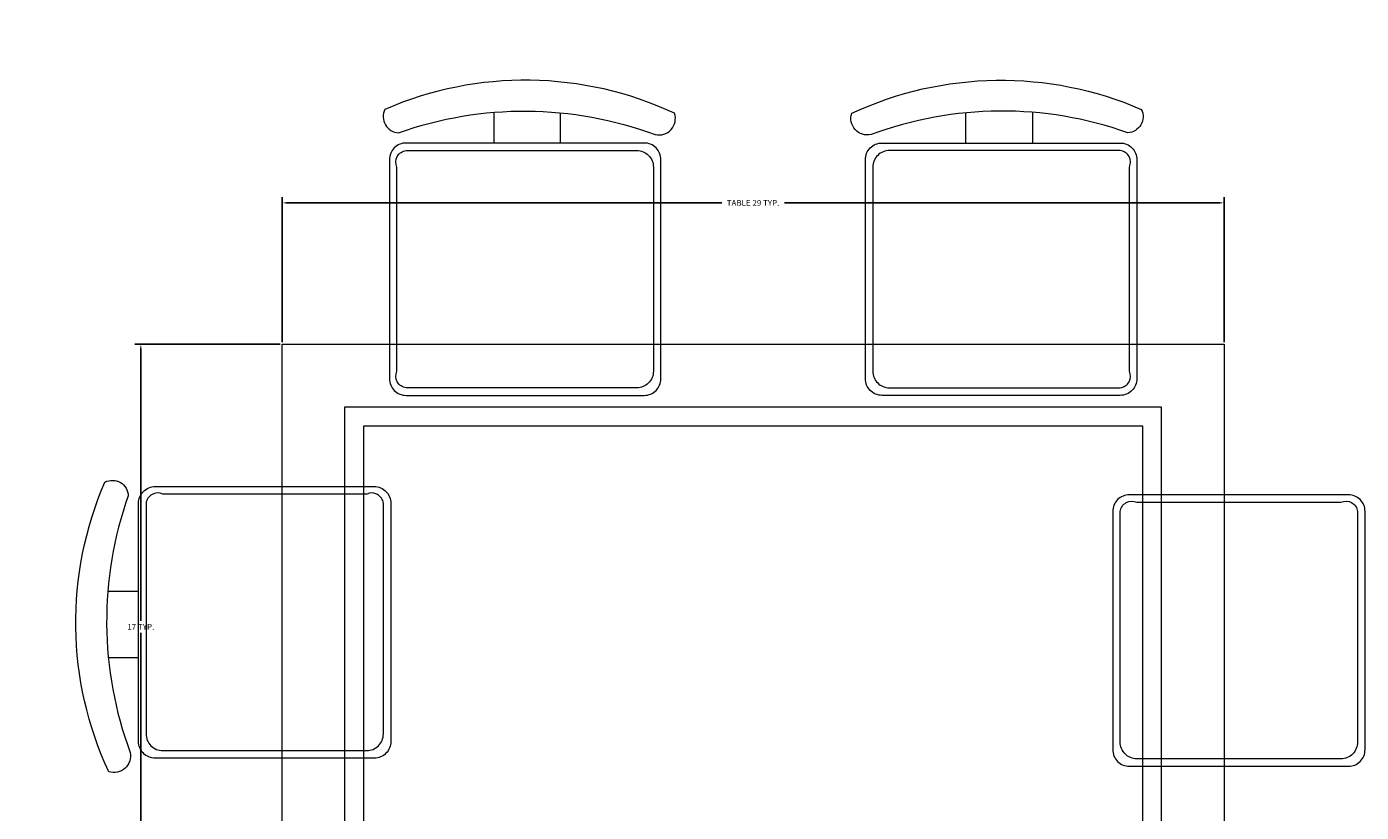
# Model space of a CAD drawing. Units: inches. Extents: x 1088 to 1703, y 668 to 1875.
# Tile 21 of 45: x 1371 to 1413, y 1648 to 1672. Entities that reach past the tile are written whole.
import ezdxf

# ---------------------------------------------------------------- set-up
doc = ezdxf.new("R2010")
doc.units = ezdxf.units.IN
doc.layers.add('A-ANNO-DIMS', color=2, linetype='Continuous', lineweight=18)
doc.layers.add('A-FURN', color=8, linetype='Continuous', lineweight=13)
doc.styles.get("Standard").update_dxf_attribs({"font": 'arial.ttf'})
doc.dimstyles.get("Standard").update_dxf_attribs({"dimtxt": 0.18, "dimasz": 0.18, "dimexe": 0.18, "dimexo": 0.0625, "dimgap": 0.09, "dimtad": 0, "dimtih": 1, "dimtoh": 1, "dimdec": 4, "dimzin": 0, "dimdsep": 46, "dimtxsty": 'Standard', "dimcen": 0.09, "dimadec": 0, "dimazin": 0, "dimtfac": 1, "dimtdec": 4, "dimtofl": 0, "dimtmove": 0, "dimatfit": 3, "dimfxl": 1, "dimtolj": 1, "dimtzin": 0, "dimarcsym": 0})

# ---------------------------------------------------------------- blocks, each defined once
blk = doc.blocks.new('TABLE-DINING-RECT')
for points in [[(0, 17.407), (29.011, 17.407), (29.011, 0), (0, 0)], [(1.934, 15.473), (27.077, 15.473), (27.077, 1.934), (1.934, 1.934)], [(2.514, 14.892), (26.497, 14.892), (26.497, 2.515), (2.514, 2.515)]]:
    blk.add_lwpolyline(points, close=True)
blk = doc.blocks.new('CHAIR-DINING')
for points in [[(7.771, 8.293, 0.414214), (7.258, 8.807), (0.513, 8.807, 0.414214), (0, 8.293), (0, 0.958, 0.414214), (0.513, 0.444), (7.258, 0.444, 0.414214), (7.771, 0.958), (7.771, 8.293)], [(8.088, 8.524, -0.175809), (8.029, 0.622, 0.578392), (8.687, 0.024, 0.214524), (8.806, 8.943, 0.552014), (8.088, 8.524, -0.065079)], [(7.771, 3.534), (8.699, 3.534, -0.064759)]]:
    blk.add_lwpolyline(points, format="xyb")
blk.add_lwpolyline([(7.54, 8.29), (7.54, 1.189, -0.414214), (7.027, 0.676), (0.744, 0.676, -0.414214), (0.231, 1.189), (0.231, 8.29, -0.512069), (0.744, 8.575), (7.027, 8.575, -0.512069)], format="xyb", close=True)
blk.add_lwpolyline([(8.716, 5.588), (7.771, 5.588)])
blk = doc.blocks.new('*D16')
at = {"layer": 'A-ANNO-DIMS', "color": 0, "lineweight": -2, "transparency": 16777216}
for p, q in [((1379.339, 1662.149), (1379.339, 1666.618)), ((1379.519, 1666.438), (1392.88, 1666.438)), ((1408.169, 1666.438), (1394.808, 1666.438)), ((1408.349, 1662.149), (1408.349, 1666.618))]:
    blk.add_line(p, q, dxfattribs=at)
at = {"layer": 'A-ANNO-DIMS', "color": 0, "transparency": 16777216}
for points in [[(1379.519, 1666.468), (1379.519, 1666.408), (1379.339, 1666.438)], [(1408.169, 1666.468), (1408.169, 1666.408), (1408.349, 1666.438)]]:
    blk.add_solid(points, dxfattribs=at)
at = {"layer": 'Defpoints', "color": 0, "transparency": 16777216}
for p in [(1408.349, 1666.438), (1379.339, 1662.086), (1408.349, 1662.086)]:
    blk.add_point(p, dxfattribs=at)
at = {"layer": 'A-ANNO-DIMS', "color": 0, "transparency": 16777216, "insert": (1393.844, 1666.438), "char_height": 0.18, "attachment_point": 5}
blk.add_mtext('\\A1;TABLE 29 TYP.', dxfattribs=at)
blk = doc.blocks.new('*D17')
at = {"layer": 'A-ANNO-DIMS', "color": 0, "lineweight": -2, "transparency": 16777216}
for p, q in [((1379.276, 1662.086), (1374.807, 1662.086)), ((1374.987, 1661.906), (1374.987, 1653.563)), ((1374.987, 1644.86), (1374.987, 1653.203)), ((1379.276, 1644.68), (1374.807, 1644.68))]:
    blk.add_line(p, q, dxfattribs=at)
at = {"layer": 'A-ANNO-DIMS', "color": 0, "transparency": 16777216}
for points in [[(1374.957, 1661.906), (1375.017, 1661.906), (1374.987, 1662.086)], [(1374.957, 1644.86), (1375.017, 1644.86), (1374.987, 1644.68)]]:
    blk.add_solid(points, dxfattribs=at)
at = {"layer": 'Defpoints', "color": 0, "transparency": 16777216}
for p in [(1374.987, 1662.086), (1379.339, 1662.086), (1379.339, 1644.68)]:
    blk.add_point(p, dxfattribs=at)
at = {"layer": 'A-ANNO-DIMS', "color": 0, "transparency": 16777216, "insert": (1374.987, 1653.383), "char_height": 0.18, "attachment_point": 5}
blk.add_mtext('\\A1;17 TYP.', dxfattribs=at)
blk = doc.blocks.new('*D38')
at = {"layer": 'A-ANNO-DIMS', "color": 0, "lineweight": -2, "transparency": 16777216}
for p, q in [((1317.345, 1736.945), (1317.345, 725.549)), ((1437.345, 1736.945), (1437.345, 725.549)), ((1317.525, 725.729), (1377.065, 725.729)), ((1437.165, 725.729), (1377.625, 725.729))]:
    blk.add_line(p, q, dxfattribs=at)
at = {"layer": 'A-ANNO-DIMS', "color": 0, "transparency": 16777216}
for points in [[(1317.525, 725.759), (1317.525, 725.699), (1317.345, 725.729)], [(1437.165, 725.759), (1437.165, 725.699), (1437.345, 725.729)]]:
    blk.add_solid(points, dxfattribs=at)
at = {"layer": 'Defpoints', "color": 0, "transparency": 16777216}
for p in [(1317.345, 1737.007), (1437.345, 1737.007), (1437.345, 725.729)]:
    blk.add_point(p, dxfattribs=at)
at = {"layer": 'A-ANNO-DIMS', "color": 0, "transparency": 16777216, "insert": (1377.345, 725.729), "char_height": 0.18, "attachment_point": 5}
blk.add_mtext('\\A1;120', dxfattribs=at)

msp = doc.modelspace()

# ---------------------------------------------------------------- linework, layer by layer
at = {"layer": 'A-FURN'}
for points in [[(1382.927, 1668.599, -0.175809), (1390.829, 1668.539, 0.578392), (1391.427, 1669.197, 0.214524), (1382.508, 1669.317, 0.552014), (1382.927, 1668.599, -0.065079)], [(1397.481, 1668.539, -0.578392), (1396.882, 1669.197, -0.214524), (1405.802, 1669.317, -0.552014), (1405.383, 1668.599, 0.175809), (1397.481, 1668.539)], [(1387.917, 1668.281), (1387.917, 1669.209, -0.064759)], [(1400.393, 1668.281), (1400.393, 1669.209, 0.064759)], [(1390.493, 1668.281), (1383.158, 1668.281, 0.414214), (1382.644, 1667.768), (1382.644, 1661.023, 0.414214), (1383.158, 1660.51), (1390.493, 1660.51, 0.414214), (1391.007, 1661.023), (1391.007, 1667.768, 0.414214), (1390.493, 1668.281)], [(1405.152, 1668.281, -0.414214), (1405.665, 1667.768), (1405.665, 1661.023, -0.414214), (1405.152, 1660.51), (1397.816, 1660.51, -0.414214), (1397.303, 1661.023), (1397.303, 1667.768, -0.414214), (1397.816, 1668.281), (1405.152, 1668.281)], [(1412.693, 1656.937, 0.414214), (1412.18, 1657.45), (1405.435, 1657.45, 0.414214), (1404.921, 1656.937), (1404.921, 1649.601, 0.414214), (1405.435, 1649.088), (1412.18, 1649.088, 0.414214), (1412.693, 1649.601), (1412.693, 1656.937)]]:
    msp.add_lwpolyline(points, format="xyb", dxfattribs=at)
for points in [[(1385.863, 1669.226), (1385.863, 1668.281)], [(1402.446, 1669.226), (1402.446, 1668.281)]]:
    msp.add_lwpolyline(points, dxfattribs=at)
for points in [[(1383.161, 1668.05), (1390.262, 1668.05, -0.414214), (1390.775, 1667.537), (1390.775, 1661.254, -0.414214), (1390.262, 1660.741), (1383.161, 1660.741, -0.512069), (1382.876, 1661.254), (1382.876, 1667.537, -0.512069)], [(1405.149, 1668.05), (1398.047, 1668.05, 0.414214), (1397.534, 1667.537), (1397.534, 1661.254, 0.414214), (1398.047, 1660.741), (1405.149, 1660.741, 0.512069), (1405.434, 1661.254), (1405.434, 1667.537, 0.512069)], [(1412.462, 1656.934), (1412.462, 1649.832, -0.414214), (1411.948, 1649.319), (1405.666, 1649.319, -0.414214), (1405.153, 1649.832), (1405.153, 1656.934, -0.512069), (1405.666, 1657.219), (1411.948, 1657.219, -0.512069)]]:
    msp.add_lwpolyline(points, format="xyb", close=True, dxfattribs=at)

# ---------------------------------------------------------------- block references
msp.add_blockref('TABLE-DINING-RECT', (1379.339, 1644.68), dxfattribs=at)
at = {"layer": 'A-FURN', "extrusion": (0, 0, -1), "zscale": -1, "rotation": 1.4787793335e-06}
msp.add_blockref('CHAIR-DINING', (-1382.689, 1648.895), dxfattribs=at)

# ---------------------------------------------------------------- dimensions: what is measured, and where the dimension line sits
at = {"layer": 'A-ANNO-DIMS'}
dim = msp.add_linear_dim(base=(1437.345, 725.729), p1=(1317.345, 1737.007), p2=(1437.345, 1737.007), dimstyle='Standard', override={"dimdec": 0, "dimlfac": 1, "dimrnd": 0, "dimzin": 0, "dimdsep": 46, "dimlunit": 2}, dxfattribs=at)
dim.commit()
dim.dimension.update_dxf_attribs({"geometry": '*D38', "text_midpoint": (1377.345, 725.729)})
dim = msp.add_linear_dim(base=(1408.349, 1666.438), p1=(1379.339, 1662.086), p2=(1408.349, 1662.086), text='TABLE <> TYP.', dimstyle='Standard', override={"dimdec": 0, "dimlfac": 1, "dimrnd": 0, "dimzin": 0, "dimdsep": 46, "dimlunit": 2}, dxfattribs=at)
dim.commit()
dim.dimension.update_dxf_attribs({"geometry": '*D16', "text_midpoint": (1393.844, 1666.438)})
dim = msp.add_linear_dim(base=(1374.987, 1662.086), p1=(1379.339, 1644.68), p2=(1379.339, 1662.086), angle=90, text='<> TYP.', dimstyle='Standard', override={"dimdec": 0, "dimlfac": 1, "dimrnd": 0, "dimzin": 0, "dimdsep": 46, "dimlunit": 2}, dxfattribs=at)
dim.commit()
dim.dimension.update_dxf_attribs({"geometry": '*D17', "text_midpoint": (1374.987, 1653.383)})

doc.saveas('drawing.dxf')
